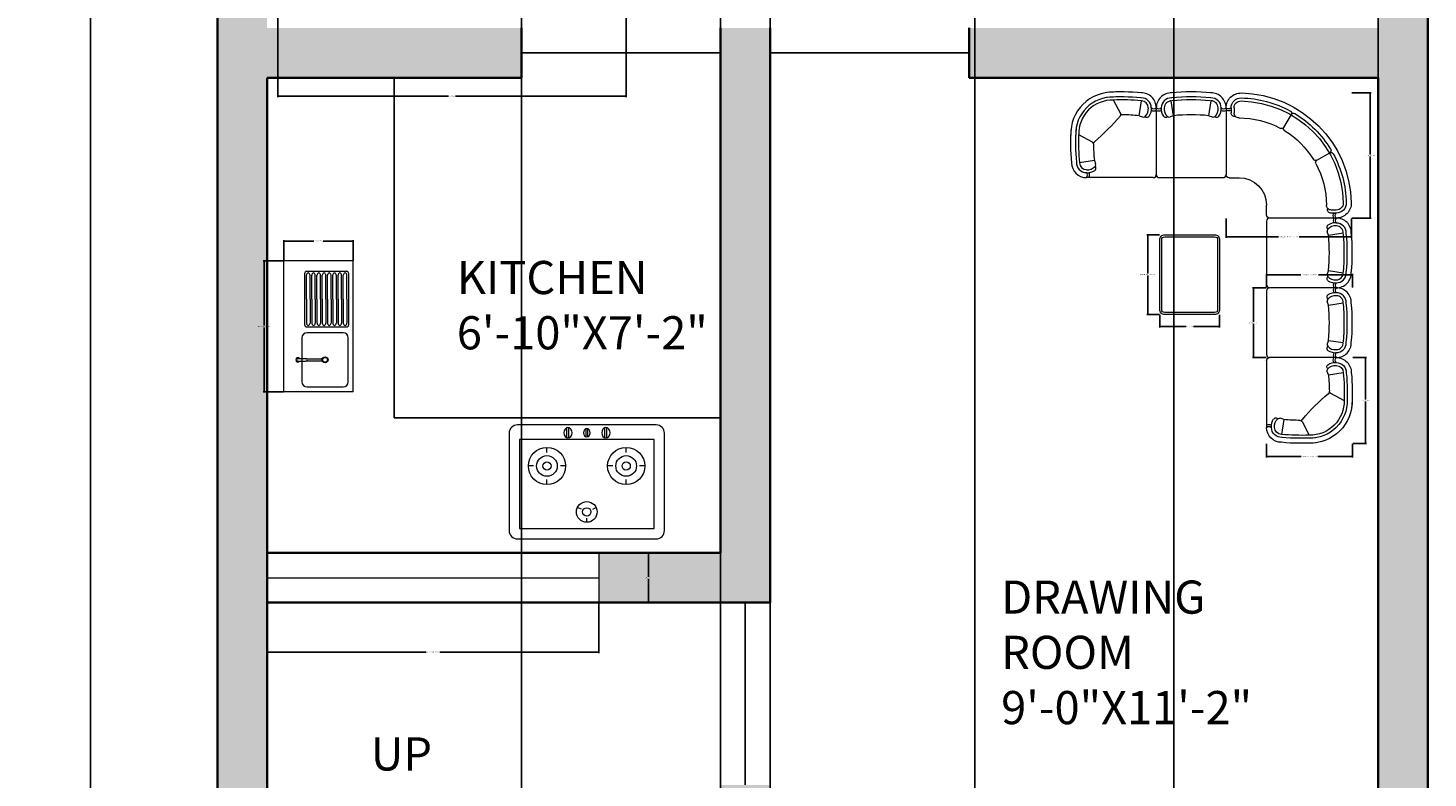
# Model space of a CAD drawing. Units: inches. Extents: x -16 to 587, y -783 to 64.
# Tile 7 of 14: x -16 to 237, y -527 to -392. Entities that reach past the tile are written whole.
import ezdxf

# ---------------------------------------------------------------- set-up
doc = ezdxf.new("R2010")
doc.units = ezdxf.units.IN
doc.header["$MEASUREMENT"] = 0
for name, color, linetype, lineweight in [('A-ANNO-DIMS', 2, 'Continuous', 18), ('A-ANNO-TEXT', 7, 'Continuous', 25), ('A-AREA-IDEN', 7, 'Continuous', 18), ('A-DOOR', 3, 'Continuous', 25), ('A-EQPM', 8, 'Continuous', 18), ('A-FLOR-CASE', 7, 'Continuous', 25), ('A-FLOR-FIXT', 9, 'Continuous', 18), ('A-FURN', 8, 'Continuous', 18), ('A-GLAZ', 4, 'Continuous', 18), ('A-WALL', 7, 'Continuous', 35), ('A-WALL-PATT', 23, 'Continuous', 13)]:
    doc.layers.add(name, color=color, linetype=linetype, lineweight=lineweight)
doc.styles.get("Standard").update_dxf_attribs({"font": 'arial.ttf'})
doc.dimstyles.get("Standard").update_dxf_attribs({"dimtxt": 0.18, "dimasz": 0.18, "dimexe": 0.18, "dimexo": 0.0625, "dimgap": 0.09, "dimtad": 0, "dimtih": 1, "dimtoh": 1, "dimdec": 0, "dimzin": 0, "dimdsep": 46, "dimlunit": 3, "dimtxsty": 'Standard', "dimcen": 0.09, "dimadec": 0, "dimazin": 0, "dimtfac": 1, "dimtdec": 0, "dimtofl": 0, "dimtmove": 0, "dimatfit": 3, "dimfxl": 1, "dimtolj": 1, "dimtzin": 0, "dimarcsym": 0})

# ---------------------------------------------------------------- blocks, each defined once
blk = doc.blocks.new('A$C707258B2')
at = {"color": 0}
for p, q in [((0.404, 0.342), (1.074, 0.342)), ((0.404, 0.292), (0.454, 0.292)), ((1.104, 0.312), (1.104, 0.212)), ((0.404, 0.262), (0.454, 0.262)), ((1.479, -0.063), (1.379, -0.063)), ((1.509, -0.763), (1.509, -0.093)), ((0.6, -0.238), (0.47, -0.313)), ((0.929, -0.567), (0.854, -0.697)), ((1.429, -0.763), (1.429, -0.713)), ((1.459, -0.763), (1.459, -0.712))]:
    blk.add_line(p, q, dxfattribs=at)
for centre, radius, start, end in [((0.404, 0.192), 0.15, 90, 181.1754), ((0.404, 0.192), 0.1, 90, 181.1754), ((0.378, 0.317), 0.0362, 316.3972, 43.6028), ((0.368, 0.317), 0.0662, 337.8298, 22.1702), ((0.455, 0.256), 0.0357, 345.4262, 90.5555), ((1.074, 0.312), 0.03, 360, 90), ((1.379, 0.212), 1.125, 181.1754, 268.8246), ((1.379, 0.212), 1.075, 181.1754, 208.6357), ((0.404, 0.192), 0.07, 90, 181.1754), ((1.379, 0.212), 1.045, 181.1754, 268.8246), ((0.454, 0.212), 0.05, 360, 90), ((1.379, 0.212), 0.875, 180, 208.4082), ((1.379, 0.212), 0.275, 180, 270), ((1.479, -0.093), 0.03, 360, 90), ((0.587, -0.216), 0.025, 300, 28.4082), ((0.612, -0.259), 0.025, 31.5918, 120), ((1.379, 0.212), 0.875, 211.5918, 238.4082), ((0.457, -0.291), 0.025, 208.6357, 300), ((0.482, -0.334), 0.025, 120, 211.3643), ((1.379, 0.212), 1.075, 211.3643, 238.6357), ((0.907, -0.555), 0.025, 330, 58.4082), ((0.951, -0.58), 0.025, 61.5918, 150), ((1.379, 0.212), 0.875, 241.5918, 270), ((0.832, -0.685), 0.025, 238.6357, 330), ((0.876, -0.71), 0.025, 150, 241.3643), ((1.379, -0.713), 0.05, 360, 90), ((1.425, -0.709), 0.0336, 354.6301, 109.3883), ((1.379, 0.212), 1.075, 241.3643, 268.8246), ((1.359, -0.763), 0.15, 268.8246, 360), ((1.359, -0.763), 0.1, 268.8246, 360), ((1.359, -0.763), 0.07, 268.8246, 360), ((1.484, -0.799), 0.0662, 67.8298, 112.1702), ((1.484, -0.789), 0.0362, 46.3972, 133.6028)]:
    blk.add_arc(centre, radius, start, end, dxfattribs=at)
blk = doc.blocks.new('A$C1352')
at = {"color": 0}
for points in [[(0.003, 0.053), (0.003, 0.553, -0.414214), (0.053, 0.603), (0.753, 0.603, -0.414214), (0.803, 0.553), (0.803, 0.053, -0.414214), (0.753, 0.003), (0.053, 0.003, -0.414214)], [(0.023, 0.053), (0.023, 0.553, -0.414214), (0.053, 0.583), (0.753, 0.583, -0.414214), (0.783, 0.553), (0.783, 0.053, -0.414214), (0.753, 0.023), (0.053, 0.023, -0.414214)]]:
    blk.add_lwpolyline(points, format="xyb", close=True, dxfattribs=at)
blk = doc.blocks.new('part 01')
at = {"color": 0}
for p, q in [((-670, 700), (0, 700)), ((30, 30), (30, 670)), ((-591, 527), (-740, 550)), ((-591, 527), (-579, 561)), ((-591, 173), (-740, 150)), ((-591, 173), (-579, 139)), ((-670, 0), (0, 0))]:
    blk.add_line(p, q, dxfattribs=at)
for centre, radius, start, end in [((-670, 550), 150, 90, 181.1754), ((-670, 550), 100, 90, 181.1754), ((-670, 550), 70, 90, 181.1754), ((-660, 518), 133, 56.0897, 95.6132), ((-696, 675), 36.2, 316.3972, 43.6028), ((-660, 518), 103, 42.0066, 95.6132), ((-706, 675), 66.2, 337.8298, 22.1702), ((-600, 607), 25, 332.9608, 56.0897), ((-625, 620), 53.2, 321.0017, 332.9608), ((-602, 570), 25, 340, 42.0066), ((0, 670), 30, 0, 90), ((1178, 350), 2008, 174.2835, 185.7165), ((1178, 350), 1958, 174.2835, 185.7165), ((1178, 350), 1928, 174.2835, 185.7165), ((1178, 350), 1778, 174.2835, 185.7165), ((-670, 150), 150, 178.8246, 270), ((-670, 150), 100, 178.8246, 270), ((-670, 150), 70, 178.8246, 270), ((-660, 182), 133, 264.3868, 303.9103), ((-660, 182), 103, 264.3868, 317.9934), ((-696, 25), 36.2, 316.3972, 43.6028), ((-706, 25), 66.2, 337.8298, 22.1702), ((-600, 93), 25, 303.9103, 27.0392), ((-602, 130), 25, 317.9934, 20), ((-625, 80), 53.2, 27.0392, 38.9983), ((0, 30), 30, 270, 0)]:
    blk.add_arc(centre, radius, start, end, dxfattribs=at)
blk = doc.blocks.new('part02')
at = {"color": 0}
for p, q in [((0, -670), (0, 0)), ((30, 30), (700, 30)), ((621, -143), (609, -109)), ((621, -143), (770, -120)), ((640, -326), (778, -399)), ((173, -591), (139, -579)), ((173, -591), (150, -740)), ((356, -610), (429, -748))]:
    blk.add_line(p, q, dxfattribs=at)
for centre, radius, start, end in [((30, 0), 30, 90, 180), ((726, 5), 56.2, 153.6122, 206.6666), ((726, 5), 36.2, 136.3972, 223.6028), ((700, -120), 150, 0, 90), ((630, -63), 25, 123.9103, 207.0392), ((655, -50), 53.2, 207.0392, 218.9983), ((632, -100), 25, 137.9934, 200), ((690, -152), 103, 84.3868, 137.9934), ((689, -151), 132, 85.4378, 123.9887), ((700, -121), 101, 357.5006, 89.858), ((700, -120), 70, 0, 90), ((-1228, -320), 2008, 357.7349, 5.7032), ((-1148, -320), 1958, 355.8657, 5.7165), ((-1148, -320), 2008, 355.818, 5.7165), ((-1148, -320), 1778, 0.3836, 5.7165), ((2220, -2190), 2454, 130.6961, 139.3039), ((439, -409), 419, 268.2181, 1.7819), ((439, -409), 369, 268.2181, 1.7819), ((439, -409), 339, 268.2181, 1.7819), ((632, -344), 20, 62, 130.6961), ((650, -308), 20, 180.3836, 242), ((25, -696), 56.2, 63.3334, 116.3878), ((25, -696), 36.2, 46.3972, 133.6028), ((150, -670), 150, 180, 271.1754), ((182, -660), 133, 146.0897, 185.6132), ((150, -670), 100, 180, 271.1754), ((93, -600), 25, 62.9608, 146.0897), ((182, -660), 103, 132.0066, 185.6132), ((150, -670), 70, 180, 270), ((80, -625), 53.2, 51.0017, 62.9608), ((130, -602), 25, 70, 132.0066), ((350, 1178), 1778, 264.2835, 269.6164), ((338, -620), 20, 28, 89.6164), ((374, -602), 20, 139.3039, 208), ((350, 1258), 2008, 264.2968, 272.2651), ((350, 1178), 2008, 264.2835, 274.182), ((350, 1178), 1958, 264.2835, 274.1343)]:
    blk.add_arc(centre, radius, start, end, dxfattribs=at)
blk = doc.blocks.new('*D6')
at = {"layer": 'A-ANNO-DIMS', "color": 0, "lineweight": -2, "transparency": 16777216}
for p, q in [((18.02, 19.45), (-5.05, 19.45)), ((-4.87, 19.27), (-4.87, -355.9)), ((-4.87, -737.37), (-4.87, -362.21)), ((18.02, -737.55), (-5.05, -737.55))]:
    blk.add_line(p, q, dxfattribs=at)
at = {"layer": 'A-ANNO-DIMS', "color": 0, "transparency": 16777216}
for points in [[(-4.9, 19.27), (-4.84, 19.27), (-4.87, 19.45)], [(-4.9, -737.37), (-4.84, -737.37), (-4.87, -737.55)]]:
    blk.add_solid(points, dxfattribs=at)
at = {"layer": 'Defpoints', "color": 0, "transparency": 16777216}
for p in [(18.08, 19.45), (-4.87, -737.55), (18.08, -737.55)]:
    blk.add_point(p, dxfattribs=at)
at = {"layer": 'A-ANNO-DIMS', "color": 0, "transparency": 16777216, "insert": (-4.87, -359.05), "char_height": 6, "attachment_point": 5}
blk.add_mtext('\\A1;63\'-1"', dxfattribs=at)
blk = doc.blocks.new('KITCHEN-SINK')
for p, q in [((12.53, 23.71), (0, 23.71)), ((0, 0), (0, 23.71)), ((12.53, 0), (12.53, 23.71)), ((3.76, 21.39), (3.76, 12.19)), ((4.1, 16.79), (4.1, 21.13)), ((4.19, 21.83), (11.32, 21.83)), ((4.75, 16.79), (4.75, 21.13)), ((5.05, 16.79), (5.05, 21.13)), ((5.7, 16.79), (5.7, 21.13)), ((6, 16.79), (6, 21.13)), ((6.65, 16.79), (6.65, 21.13)), ((6.96, 16.79), (6.96, 21.13)), ((7.6, 16.79), (7.6, 21.13)), ((7.91, 16.79), (7.91, 21.13)), ((8.56, 16.79), (8.56, 21.13)), ((8.86, 16.79), (8.86, 21.13)), ((9.51, 16.79), (9.51, 21.13)), ((9.81, 16.79), (9.81, 21.13)), ((10.46, 16.79), (10.46, 21.13)), ((10.76, 16.79), (10.76, 21.13)), ((11.41, 16.79), (11.41, 21.13)), ((11.75, 12.19), (11.75, 21.39)), ((4.1, 16.79), (4.1, 12.45)), ((4.75, 16.79), (4.75, 12.45)), ((5.05, 16.79), (5.05, 12.45)), ((5.7, 16.79), (5.7, 12.45)), ((6, 16.79), (6, 12.45)), ((6.65, 16.79), (6.65, 12.45)), ((6.96, 16.79), (6.96, 12.45)), ((7.6, 16.79), (7.6, 12.45)), ((7.91, 16.79), (7.91, 12.45)), ((8.56, 16.79), (8.56, 12.45)), ((8.86, 16.79), (8.86, 12.45)), ((9.51, 16.79), (9.51, 12.45)), ((9.81, 16.79), (9.81, 12.45)), ((10.46, 16.79), (10.46, 12.45)), ((10.76, 16.79), (10.76, 12.45)), ((11.41, 16.79), (11.41, 12.45)), ((4.19, 11.76), (11.32, 11.76)), ((10.73, 10.7), (4.21, 10.7)), ((3.28, 9.77), (3.28, 6.06)), ((11.66, 1.84), (11.66, 9.77)), ((3.28, 5.95), (3.28, 1.84)), ((4.21, 0.91), (10.73, 0.91)), ((12.53, 0), (0, 0))]:
    blk.add_line(p, q)
for points in [[(2.55, 6.06), (3.98, 6.06)], [(2.55, 5.54), (3.98, 5.54)], [(4.14, 6), (6.76, 6)], [(4.14, 5.61), (6.76, 5.61)]]:
    blk.add_lwpolyline(points)
for radius in [0.54, 0.432]:
    blk.add_circle((7.47, 5.8), radius)
for centre, radius, start, end in [((4.19, 21.39), 0.432, 90, 180), ((4.53, 21.13), 0.432, 104.4903, 180), ((4.32, 21.13), 0.432, 0, 75.5097), ((5.48, 21.13), 0.432, 104.4903, 180), ((5.27, 21.13), 0.432, 0, 75.5097), ((6.44, 21.13), 0.432, 104.4903, 180), ((6.22, 21.13), 0.432, 0, 75.5097), ((7.39, 21.13), 0.432, 104.4903, 180), ((7.17, 21.13), 0.432, 0, 75.5097), ((8.34, 21.13), 0.432, 104.4903, 180), ((8.12, 21.13), 0.432, 0, 75.5097), ((9.29, 21.13), 0.432, 104.4903, 180), ((9.07, 21.13), 0.432, 0, 75.5097), ((10.24, 21.13), 0.432, 104.4903, 180), ((10.03, 21.13), 0.432, 0, 75.5097), ((11.19, 21.13), 0.432, 104.4903, 180), ((10.98, 21.13), 0.432, 0, 75.5097), ((11.32, 21.39), 0.432, 0, 90), ((4.21, 9.77), 0.933, 90, 180), ((4.19, 12.19), 0.432, 180, 270), ((4.53, 12.45), 0.432, 180, 255.5097), ((4.32, 12.45), 0.432, 284.4903, 0), ((5.48, 12.45), 0.432, 180, 255.5097), ((5.27, 12.45), 0.432, 284.4903, 0), ((6.44, 12.45), 0.432, 180, 255.5097), ((6.22, 12.45), 0.432, 284.4903, 0), ((7.39, 12.45), 0.432, 180, 255.5097), ((7.17, 12.45), 0.432, 284.4903, 0), ((8.34, 12.45), 0.432, 180, 255.5097), ((8.12, 12.45), 0.432, 284.4903, 0), ((9.29, 12.45), 0.432, 180, 255.5097), ((9.07, 12.45), 0.432, 284.4903, 0), ((10.24, 12.45), 0.432, 180, 255.5097), ((10.03, 12.45), 0.432, 284.4903, 0), ((10.73, 9.77), 0.933, 0, 90), ((11.19, 12.45), 0.432, 180, 255.5097), ((10.98, 12.45), 0.432, 284.4903, 0), ((11.32, 12.19), 0.432, 270, 0), ((2.55, 5.8), 0.388, 41.9018, 318.0982), ((2.55, 5.8), 0.259, 90, 270), ((3.97, 5.8), 0.259, 272.2198, 87.7802), ((6.78, 5.8), 0.195, 264.9463, 95.0537), ((4.21, 1.84), 0.933, 180, 270), ((10.73, 1.84), 0.933, 270, 0)]:
    blk.add_arc(centre, radius, start, end)
blk = doc.blocks.new('COOKTOP-THREE-BURNER')
for p, q in [((26.61, 20.61), (1.5, 20.61)), ((0, 19.11), (0, 1.5)), ((26.23, 17.99), (1.87, 17.99)), ((1.87, 17.99), (1.87, 1.87)), ((10.46, 18.28), (10.46, 20.15)), ((10.83, 18.28), (10.83, 20.15)), ((13.92, 18.45), (13.92, 19.97)), ((14.22, 18.45), (14.22, 19.97)), ((17.32, 18.28), (17.32, 20.15)), ((17.7, 18.28), (17.7, 20.15)), ((26.23, 1.87), (26.23, 17.99)), ((28.11, 1.5), (28.11, 19.11)), ((6.85, 15.63), (6.85, 16.56)), ((21.18, 15.63), (21.18, 16.56)), ((4.42, 13.19), (3.48, 13.19)), ((10.23, 13.19), (9.29, 13.19)), ((18.74, 13.19), (17.8, 13.19)), ((24.55, 13.19), (23.61, 13.19)), ((6.85, 9.82), (6.85, 10.76)), ((21.18, 9.82), (21.18, 10.76)), ((12.37, 5.69), (13.06, 5.41)), ((15.74, 5.69), (15.08, 5.34)), ((14.05, 3), (14.05, 3.75)), ((1.5, 0), (26.61, 0)), ((1.87, 1.87), (26.23, 1.87))]:
    blk.add_line(p, q)
for centre, radius in [((6.85, 13.19), 3.37), ((21.18, 13.19), 3.37), ((6.85, 13.19), 1.87), ((6.85, 13.19), 0.75), ((21.18, 13.19), 1.87), ((21.18, 13.19), 0.75), ((14.05, 4.88), 1.87), ((14.05, 4.88), 0.75)]:
    blk.add_circle(centre, radius)
for centre, start, end in [((1.5, 19.11), 90, 180), ((26.61, 19.11), 0, 90), ((1.5, 1.5), 180, 270), ((26.61, 1.5), 270, 0)]:
    blk.add_arc(centre, 1.5, start, end)
at = {"extrusion": (0, 0, -1)}
for centre, major_axis in [((10.65, 19.21), (0, 0.937)), ((14.07, 19.21), (0, 0.759)), ((17.51, 19.21), (0, 0.937))]:
    blk.add_ellipse(centre, major_axis=major_axis, ratio=0.802399, dxfattribs=at)
blk = doc.blocks.new('WIN-60')
for p, q in [((0, 9), (60, 9)), ((0, 0), (0, 9)), ((60, 9), (60, 0)), ((0, 4.5), (60, 4.5)), ((60, 0), (0, 0))]:
    blk.add_line(p, q)
blk = doc.blocks.new('*D20')
at = {"layer": 'A-ANNO-DIMS', "color": 0, "lineweight": -2, "transparency": 16777216}
for p, q in [((207.87, -438.52), (207.87, -436.07)), ((208.05, -436.25), (214.07, -436.25)), ((223.26, -436.25), (217.25, -436.25)), ((223.44, -438.52), (223.44, -436.07))]:
    blk.add_line(p, q, dxfattribs=at)
at = {"layer": 'A-ANNO-DIMS', "color": 0, "transparency": 16777216}
for points in [[(208.05, -436.22), (208.05, -436.28), (207.87, -436.25)], [(223.26, -436.22), (223.26, -436.28), (223.44, -436.25)]]:
    blk.add_solid(points, dxfattribs=at)
at = {"layer": 'Defpoints', "color": 0, "transparency": 16777216}
for p in [(207.87, -436.25), (207.87, -438.58), (223.44, -438.58)]:
    blk.add_point(p, dxfattribs=at)
at = {"layer": 'A-ANNO-DIMS', "color": 0, "transparency": 16777216, "insert": (215.66, -436.25), "char_height": 0.18, "attachment_point": 5}
blk.add_mtext('\\A1;SOFA SEAT 1\'-3 1/2" TYP.', dxfattribs=at)
blk = doc.blocks.new('*D21')
at = {"layer": 'A-ANNO-DIMS', "color": 0, "lineweight": -2, "transparency": 16777216}
for p, q in [((207.81, -438.58), (205.35, -438.58)), ((205.53, -438.76), (205.53, -444.72)), ((205.53, -451.03), (205.53, -445.08)), ((207.81, -451.21), (205.35, -451.21))]:
    blk.add_line(p, q, dxfattribs=at)
at = {"layer": 'A-ANNO-DIMS', "color": 0, "transparency": 16777216}
for points in [[(205.5, -438.76), (205.56, -438.76), (205.53, -438.58)], [(205.5, -451.03), (205.56, -451.03), (205.53, -451.21)]]:
    blk.add_solid(points, dxfattribs=at)
at = {"layer": 'Defpoints', "color": 0, "transparency": 16777216}
for p in [(207.87, -438.58), (205.53, -451.21), (207.87, -451.21)]:
    blk.add_point(p, dxfattribs=at)
at = {"layer": 'A-ANNO-DIMS', "color": 0, "transparency": 16777216, "insert": (205.53, -444.9), "char_height": 0.18, "attachment_point": 5}
blk.add_mtext('\\A1;1\'-0 1/2" TYP.', dxfattribs=at)
blk = doc.blocks.new('*D22')
at = {"layer": 'A-ANNO-DIMS', "color": 0, "lineweight": -2, "transparency": 16777216}
for p, q in [((207.87, -466.85), (207.87, -469.3)), ((223.44, -466.85), (223.44, -469.3)), ((208.05, -469.12), (214.13, -469.12)), ((223.26, -469.12), (217.18, -469.12))]:
    blk.add_line(p, q, dxfattribs=at)
at = {"layer": 'A-ANNO-DIMS', "color": 0, "transparency": 16777216}
for points in [[(208.05, -469.09), (208.05, -469.15), (207.87, -469.12)], [(223.26, -469.09), (223.26, -469.15), (223.44, -469.12)]]:
    blk.add_solid(points, dxfattribs=at)
at = {"layer": 'Defpoints', "color": 0, "transparency": 16777216}
for p in [(207.87, -466.78), (223.44, -466.78), (207.87, -469.12)]:
    blk.add_point(p, dxfattribs=at)
at = {"layer": 'A-ANNO-DIMS', "color": 0, "transparency": 16777216, "insert": (215.65, -469.12), "char_height": 0.18, "attachment_point": 5}
blk.add_mtext('\\A1;SOFA END 1\'-3 1/2" TYP.', dxfattribs=at)
blk = doc.blocks.new('*D23')
at = {"layer": 'A-ANNO-DIMS', "color": 0, "lineweight": -2, "transparency": 16777216}
for p, q in [((223.5, -451.21), (225.95, -451.21)), ((225.77, -451.39), (225.77, -458.82)), ((225.77, -466.6), (225.77, -459.18)), ((223.5, -466.78), (225.95, -466.78))]:
    blk.add_line(p, q, dxfattribs=at)
at = {"layer": 'A-ANNO-DIMS', "color": 0, "transparency": 16777216}
for points in [[(225.74, -451.39), (225.8, -451.39), (225.77, -451.21)], [(225.74, -466.6), (225.8, -466.6), (225.77, -466.78)]]:
    blk.add_solid(points, dxfattribs=at)
at = {"layer": 'Defpoints', "color": 0, "transparency": 16777216}
for p in [(223.44, -451.21), (223.44, -466.78), (225.77, -466.78)]:
    blk.add_point(p, dxfattribs=at)
at = {"layer": 'A-ANNO-DIMS', "color": 0, "transparency": 16777216, "insert": (225.77, -459), "char_height": 0.18, "attachment_point": 5}
blk.add_mtext('\\A1;1\'-3 1/2" TYP.', dxfattribs=at)
blk = doc.blocks.new('*D24')
at = {"layer": 'A-ANNO-DIMS', "color": 0, "lineweight": -2, "transparency": 16777216}
for p, q in [((200.56, -426.02), (200.56, -429.53)), ((223.22, -426.02), (223.22, -429.53)), ((200.74, -429.35), (210.02, -429.35)), ((223.04, -429.35), (213.76, -429.35))]:
    blk.add_line(p, q, dxfattribs=at)
at = {"layer": 'A-ANNO-DIMS', "color": 0, "transparency": 16777216}
for points in [[(200.74, -429.32), (200.74, -429.38), (200.56, -429.35)], [(223.04, -429.32), (223.04, -429.38), (223.22, -429.35)]]:
    blk.add_solid(points, dxfattribs=at)
at = {"layer": 'Defpoints', "color": 0, "transparency": 16777216}
for p in [(200.56, -425.95), (223.22, -425.95), (200.56, -429.35)]:
    blk.add_point(p, dxfattribs=at)
at = {"layer": 'A-ANNO-DIMS', "color": 0, "transparency": 16777216, "insert": (211.89, -429.35), "char_height": 0.18, "attachment_point": 5}
blk.add_mtext('\\A1;SOFA CORNER 1\'-10 1/2" TYP.', dxfattribs=at)
blk = doc.blocks.new('*D25')
at = {"layer": 'A-ANNO-DIMS', "color": 0, "lineweight": -2, "transparency": 16777216}
for p, q in [((223.28, -403.3), (226.8, -403.3)), ((226.62, -403.48), (226.62, -414.44)), ((226.62, -425.77), (226.62, -414.81)), ((223.28, -425.95), (226.8, -425.95))]:
    blk.add_line(p, q, dxfattribs=at)
at = {"layer": 'A-ANNO-DIMS', "color": 0, "transparency": 16777216}
for points in [[(226.59, -403.48), (226.65, -403.48), (226.62, -403.3)], [(226.59, -425.77), (226.65, -425.77), (226.62, -425.95)]]:
    blk.add_solid(points, dxfattribs=at)
at = {"layer": 'Defpoints', "color": 0, "transparency": 16777216}
for p in [(223.22, -403.3), (223.22, -425.95), (226.62, -425.95)]:
    blk.add_point(p, dxfattribs=at)
at = {"layer": 'A-ANNO-DIMS', "color": 0, "transparency": 16777216, "insert": (226.62, -414.63), "char_height": 0.18, "attachment_point": 5}
blk.add_mtext('\\A1;1\'-10 1/2" TYP.', dxfattribs=at)
blk = doc.blocks.new('*D26')
at = {"layer": 'A-ANNO-DIMS', "color": 0, "lineweight": -2, "transparency": 16777216}
for p, q in [((188.49, -428.98), (186.21, -428.98)), ((186.39, -429.16), (186.39, -436.01)), ((186.39, -443.23), (186.39, -436.38)), ((188.49, -443.41), (186.21, -443.41))]:
    blk.add_line(p, q, dxfattribs=at)
at = {"layer": 'A-ANNO-DIMS', "color": 0, "transparency": 16777216}
for points in [[(186.36, -429.16), (186.42, -429.16), (186.39, -428.98)], [(186.36, -443.23), (186.42, -443.23), (186.39, -443.41)]]:
    blk.add_solid(points, dxfattribs=at)
at = {"layer": 'Defpoints', "color": 0, "transparency": 16777216}
for p in [(188.55, -428.98), (186.39, -443.41), (188.55, -443.41)]:
    blk.add_point(p, dxfattribs=at)
at = {"layer": 'A-ANNO-DIMS', "color": 0, "transparency": 16777216, "insert": (186.39, -436.2), "char_height": 0.18, "attachment_point": 5}
blk.add_mtext('\\A1;SIDE TABLE 1\'-2 1/2" TYP.', dxfattribs=at)
blk = doc.blocks.new('*D27')
at = {"layer": 'A-ANNO-DIMS', "color": 0, "lineweight": -2, "transparency": 16777216}
for p, q in [((188.55, -443.48), (188.55, -445.76)), ((188.73, -445.58), (193.26, -445.58)), ((199.2, -445.58), (194.68, -445.58)), ((199.38, -443.48), (199.38, -445.76))]:
    blk.add_line(p, q, dxfattribs=at)
at = {"layer": 'A-ANNO-DIMS', "color": 0, "transparency": 16777216}
for points in [[(188.73, -445.55), (188.73, -445.61), (188.55, -445.58)], [(199.2, -445.55), (199.2, -445.61), (199.38, -445.58)]]:
    blk.add_solid(points, dxfattribs=at)
at = {"layer": 'Defpoints', "color": 0, "transparency": 16777216}
for p in [(188.55, -443.41), (199.38, -443.41), (199.38, -445.58)]:
    blk.add_point(p, dxfattribs=at)
at = {"layer": 'A-ANNO-DIMS', "color": 0, "transparency": 16777216, "insert": (193.97, -445.58), "char_height": 0.18, "attachment_point": 5}
blk.add_mtext('\\A1;0\'-11" TYP.', dxfattribs=at)
blk = doc.blocks.new('*D37')
at = {"layer": 'A-ANNO-DIMS', "color": 0, "lineweight": -2, "transparency": 16777216}
for p, q in [((29.02, -389.37), (29.02, -404.05)), ((92.05, -389.37), (92.05, -404.05)), ((29.2, -403.87), (59.9, -403.87)), ((91.87, -403.87), (61.18, -403.87))]:
    blk.add_line(p, q, dxfattribs=at)
at = {"layer": 'A-ANNO-DIMS', "color": 0, "transparency": 16777216}
for points in [[(29.2, -403.84), (29.2, -403.9), (29.02, -403.87)], [(91.87, -403.84), (91.87, -403.9), (92.05, -403.87)]]:
    blk.add_solid(points, dxfattribs=at)
at = {"layer": 'Defpoints', "color": 0, "transparency": 16777216}
for p in [(29.02, -389.31), (92.05, -389.31), (92.05, -403.87)]:
    blk.add_point(p, dxfattribs=at)
at = {"layer": 'A-ANNO-DIMS', "color": 0, "transparency": 16777216, "insert": (60.54, -403.87), "char_height": 0.18, "attachment_point": 5}
blk.add_mtext('\\A1;5\'-3" TYP.', dxfattribs=at)
blk = doc.blocks.new('*D38')
at = {"layer": 'A-ANNO-DIMS', "color": 0, "lineweight": -2, "transparency": 16777216}
for p, q in [((30.03, -433.72), (26.35, -433.72)), ((26.53, -433.9), (26.53, -445.39)), ((26.53, -457.24), (26.53, -445.75)), ((30.03, -457.42), (26.35, -457.42))]:
    blk.add_line(p, q, dxfattribs=at)
at = {"layer": 'A-ANNO-DIMS', "color": 0, "transparency": 16777216}
for points in [[(26.5, -433.9), (26.56, -433.9), (26.53, -433.72)], [(26.5, -457.24), (26.56, -457.24), (26.53, -457.42)]]:
    blk.add_solid(points, dxfattribs=at)
at = {"layer": 'Defpoints', "color": 0, "transparency": 16777216}
for p in [(26.53, -433.72), (30.09, -433.72), (30.09, -457.42)]:
    blk.add_point(p, dxfattribs=at)
at = {"layer": 'A-ANNO-DIMS', "color": 0, "transparency": 16777216, "insert": (26.53, -445.57), "char_height": 0.18, "attachment_point": 5}
blk.add_mtext('\\A1;SINK 1\'-11 1/2" TYP.', dxfattribs=at)
blk = doc.blocks.new('*D39')
at = {"layer": 'A-ANNO-DIMS', "color": 0, "lineweight": -2, "transparency": 16777216}
for p, q in [((30.09, -433.65), (30.09, -429.98)), ((30.27, -430.16), (35.52, -430.16)), ((42.44, -430.16), (37.2, -430.16)), ((42.62, -433.65), (42.62, -429.98))]:
    blk.add_line(p, q, dxfattribs=at)
at = {"layer": 'A-ANNO-DIMS', "color": 0, "transparency": 16777216}
for points in [[(30.27, -430.13), (30.27, -430.19), (30.09, -430.16)], [(42.44, -430.13), (42.44, -430.19), (42.62, -430.16)]]:
    blk.add_solid(points, dxfattribs=at)
at = {"layer": 'Defpoints', "color": 0, "transparency": 16777216}
for p in [(42.62, -430.16), (30.09, -433.72), (42.62, -433.72)]:
    blk.add_point(p, dxfattribs=at)
at = {"layer": 'A-ANNO-DIMS', "color": 0, "transparency": 16777216, "insert": (36.36, -430.16), "char_height": 0.18, "attachment_point": 5}
blk.add_mtext('\\A1;1\'-0 1/2" TYP.', dxfattribs=at)
blk = doc.blocks.new('*D46')
at = {"layer": 'A-ANNO-DIMS', "color": 0, "lineweight": -2, "transparency": 16777216}
for p, q in [((27.08, -495.62), (27.08, -504.73)), ((87.08, -495.62), (87.08, -504.73)), ((27.26, -504.55), (55.85, -504.55)), ((86.9, -504.55), (58.31, -504.55))]:
    blk.add_line(p, q, dxfattribs=at)
at = {"layer": 'A-ANNO-DIMS', "color": 0, "transparency": 16777216}
for points in [[(27.26, -504.52), (27.26, -504.58), (27.08, -504.55)], [(86.9, -504.52), (86.9, -504.58), (87.08, -504.55)]]:
    blk.add_solid(points, dxfattribs=at)
at = {"layer": 'Defpoints', "color": 0, "transparency": 16777216}
for p in [(27.08, -495.55), (87.08, -495.55), (87.08, -504.55)]:
    blk.add_point(p, dxfattribs=at)
at = {"layer": 'A-ANNO-DIMS', "color": 0, "transparency": 16777216, "insert": (57.08, -504.55), "char_height": 0.18, "attachment_point": 5}
blk.add_mtext('\\A1;WINDOW 5\'-0" TYP.', dxfattribs=at)
blk = doc.blocks.new('*D47')
at = {"layer": 'A-ANNO-DIMS', "color": 0, "lineweight": -2, "transparency": 16777216}
for p, q in [((87.15, -486.55), (96.26, -486.55)), ((96.08, -486.73), (96.08, -490.87)), ((96.08, -495.37), (96.08, -491.24)), ((87.15, -495.55), (96.26, -495.55))]:
    blk.add_line(p, q, dxfattribs=at)
at = {"layer": 'A-ANNO-DIMS', "color": 0, "transparency": 16777216}
for points in [[(96.05, -486.73), (96.11, -486.73), (96.08, -486.55)], [(96.05, -495.37), (96.11, -495.37), (96.08, -495.55)]]:
    blk.add_solid(points, dxfattribs=at)
at = {"layer": 'Defpoints', "color": 0, "transparency": 16777216}
for p in [(87.08, -486.55), (96.08, -486.55), (87.08, -495.55)]:
    blk.add_point(p, dxfattribs=at)
at = {"layer": 'A-ANNO-DIMS', "color": 0, "transparency": 16777216, "insert": (96.08, -491.05), "char_height": 0.18, "attachment_point": 5}
blk.add_mtext('\\A1;0\'-9" TYP.', dxfattribs=at)
blk = doc.blocks.new('*D56')
at = {"layer": 'A-ANNO-DIMS', "color": 0, "lineweight": -2, "transparency": 16777216}
for p, q in [((118.08, -728.49), (118.08, 63.78)), ((118.26, 63.6), (172.75, 63.6)), ((227.9, 63.6), (173.41, 63.6)), ((228.08, -728.49), (228.08, 63.78))]:
    blk.add_line(p, q, dxfattribs=at)
at = {"layer": 'A-ANNO-DIMS', "color": 0, "transparency": 16777216}
for points in [[(118.26, 63.63), (118.26, 63.57), (118.08, 63.6)], [(227.9, 63.63), (227.9, 63.57), (228.08, 63.6)]]:
    blk.add_solid(points, dxfattribs=at)
at = {"layer": 'Defpoints', "color": 0, "transparency": 16777216}
for p in [(228.08, 63.6), (118.08, -728.55), (228.08, -728.55)]:
    blk.add_point(p, dxfattribs=at)
at = {"layer": 'A-ANNO-DIMS', "color": 0, "transparency": 16777216, "insert": (173.08, 63.6), "char_height": 0.18, "attachment_point": 5}
blk.add_mtext('\\A1;9\'-2"', dxfattribs=at)
blk = doc.blocks.new('*D57')
at = {"layer": 'A-ANNO-DIMS', "color": 0, "lineweight": -2, "transparency": 16777216}
for p, q in [((155.08, -534.49), (155.08, 63.78)), ((155.26, 63.6), (172.75, 63.6)), ((190.9, 63.6), (173.41, 63.6)), ((191.08, -534.49), (191.08, 63.78))]:
    blk.add_line(p, q, dxfattribs=at)
at = {"layer": 'A-ANNO-DIMS', "color": 0, "transparency": 16777216}
for points in [[(155.26, 63.63), (155.26, 63.57), (155.08, 63.6)], [(190.9, 63.63), (190.9, 63.57), (191.08, 63.6)]]:
    blk.add_solid(points, dxfattribs=at)
at = {"layer": 'Defpoints', "color": 0, "transparency": 16777216}
for p in [(191.08, 63.6), (155.08, -534.55), (191.08, -534.55)]:
    blk.add_point(p, dxfattribs=at)
at = {"layer": 'A-ANNO-DIMS', "color": 0, "transparency": 16777216, "insert": (173.08, 63.6), "char_height": 0.18, "attachment_point": 5}
blk.add_mtext('\\A1;3\'-0"', dxfattribs=at)
blk = doc.blocks.new('*D58')
at = {"layer": 'A-ANNO-DIMS', "color": 0, "lineweight": -2, "transparency": 16777216}
for p, q in [((73.08, -663.49), (73.08, 63.78)), ((73.26, 63.6), (90.75, 63.6)), ((108.9, 63.6), (91.41, 63.6)), ((109.08, -667.99), (109.08, 63.78))]:
    blk.add_line(p, q, dxfattribs=at)
at = {"layer": 'A-ANNO-DIMS', "color": 0, "transparency": 16777216}
for points in [[(73.26, 63.63), (73.26, 63.57), (73.08, 63.6)], [(108.9, 63.63), (108.9, 63.57), (109.08, 63.6)]]:
    blk.add_solid(points, dxfattribs=at)
at = {"layer": 'Defpoints', "color": 0, "transparency": 16777216}
for p in [(109.08, 63.6), (73.08, -663.55), (109.08, -668.05)]:
    blk.add_point(p, dxfattribs=at)
at = {"layer": 'A-ANNO-DIMS', "color": 0, "transparency": 16777216, "insert": (91.08, 63.6), "char_height": 0.18, "attachment_point": 5}
blk.add_mtext('\\A1;3\'-0"', dxfattribs=at)

msp = doc.modelspace()

# ---------------------------------------------------------------- hatches: boundary and pattern name
at = {"layer": 'A-WALL-PATT'}
h = msp.add_hatch(color=256, dxfattribs=at)
h.dxf.hatch_style = 1
h.paths.add_polyline_path([(137.08, -543.55), (137.08, -534.55), (118.08, -534.55), (118.08, -528.55), (109.08, -528.55), (109.08, -534.55), (109.08, -672.55), (118.08, -672.55), (118.08, -543.55)], flags=17)
h.paths.add_polyline_path([(27.08, -663.55), (27.08, -400.55), (73.08, -400.55), (73.08, -391.55), (27.08, -391.55), (27.08, 10.45), (48.75, 10.45), (171.08, 10.45), (171.08, -17.55), (180.08, -17.55), (180.08, 10.45), (228.08, 10.45), (228.08, -262.55), (206.41, -262.55), (118.08, -262.55), (118.08, -271.55), (228.08, -271.55), (228.08, -391.55), (154.08, -391.55), (154.08, -400.55), (228.08, -400.55), (228.08, -534.55), (209.08, -534.55), (209.08, -543.55), (237.08, -543.55), (237.08, 19.45), (18.08, 19.45), (18.08, -672.55), (73.08, -672.55), (73.08, -663.55)])
h.paths.add_polyline_path([(109.08, -486.55), (87.08, -486.55), (87.08, -495.55), (118.08, -495.55), (118.08, -400.55), (118.08, -391.55), (109.08, -391.55), (109.08, -400.55)], flags=17)

# ---------------------------------------------------------------- linework, layer by layer
at = {"layer": 'A-DOOR'}
for p, q in [((73.08, -396.05), (109.08, -396.05)), ((118.08, -396.05), (154.08, -396.05)), ((113.58, -528.55), (113.58, -495.55))]:
    msp.add_line(p, q, dxfattribs=at)
at = {"layer": 'A-FLOR-CASE'}
for p, q in [((50.08, -400.55), (50.08, -462.09)), ((50.08, -462.09), (109.08, -462.09))]:
    msp.add_line(p, q, dxfattribs=at)
at = {"layer": 'A-WALL'}
for p, q in [((18.08, 19.45), (18.08, -737.55)), ((237.08, 19.45), (237.08, -737.55)), ((73.08, -391.55), (73.08, -400.55)), ((109.08, -400.55), (109.08, -391.55)), ((118.08, -400.55), (118.08, -391.55)), ((154.08, -391.55), (154.08, -400.55)), ((27.08, -400.55), (73.08, -400.55)), ((27.08, -400.55), (27.08, -663.55)), ((109.08, -400.55), (109.08, -486.55)), ((118.08, -400.55), (118.08, -495.55)), ((154.08, -400.55), (228.08, -400.55)), ((228.08, -400.55), (228.08, -534.55)), ((27.08, -486.55), (109.08, -486.55)), ((27.08, -495.55), (118.08, -495.55))]:
    msp.add_line(p, q, dxfattribs=at)

# ---------------------------------------------------------------- block references
at = {"layer": 'A-EQPM'}
msp.add_blockref('COOKTOP-THREE-BURNER', (70.85, -484.02), dxfattribs=at)
at = {"layer": 'A-FLOR-FIXT'}
msp.add_blockref('KITCHEN-SINK', (30.09, -457.42), dxfattribs=at)
at = {"layer": 'A-FURN', "ltscale": 0.03}
for name, p, xscale, yscale, zscale, rotation in [('part02', (187.93, -418.1), 0.0180440482994306, 0.0180440482994306, 0.0180440482994306, 180), ('part 01', (187.93, -418.1), 0.0180440482994306, 0.0180440482994306, 0.0180440482994306, 270), ('A$C707258B2', (206.73, -398.73), -18.04404829943058, 18.04404829943058, 18.04404829943058, 89.9999999999967), ('part 01', (208.41, -425.95), 0.0180440482994306, 0.0180440482994306, 0.0180440482994306, 180), ('A$C1352', (188.5, -428.93), 18.04404829943058, 18.04404829943058, 18.04404829943058, 270), ('part 01', (208.41, -438.58), 0.0180440482994306, 0.0180440482994306, 0.0180440482994306, 180), ('part02', (208.41, -451.21), -0.0180440482994306, 0.0180440482994306, 0.0180440482994306, 89.9999999999967)]:
    msp.add_blockref(name, p, dxfattribs=dict(at, xscale=xscale, yscale=yscale, zscale=zscale, rotation=rotation))
at = {"layer": 'A-GLAZ'}
msp.add_blockref('WIN-60', (27.08, -495.56), dxfattribs=at)

# ---------------------------------------------------------------- texts
at = {"layer": 'A-ANNO-TEXT', "insert": (45.82, -519.95), "char_height": 6, "attachment_point": 1}
msp.add_mtext('UP', dxfattribs=at)
at = {"layer": 'A-AREA-IDEN', "char_height": 6, "attachment_point": 1}
for s, insert in [('KITCHEN\\P6\'-10"X7\'-2"', (61.39, -433.72)), ('DRAWING\\PROOM\\P9\'-0"X11\'-2"', (159.86, -491.56))]:
    msp.add_mtext(s, dxfattribs=dict(at, insert=insert))

# ---------------------------------------------------------------- dimensions: what is measured, and where the dimension line sits
at = {"layer": 'A-ANNO-DIMS'}
for base, p1, p2, picture, middle in [((109.08, 63.6), (73.08, -663.55), (109.08, -668.05), '*D58', (91.08, 63.6)), ((228.08, 63.6), (118.08, -728.55), (228.08, -728.55), '*D56', (173.08, 63.6)), ((191.08, 63.6), (155.08, -534.55), (191.08, -534.55), '*D57', (173.08, 63.6))]:
    dim = msp.add_linear_dim(base=base, p1=p1, p2=p2, dimstyle='Standard', override={"dimdec": 1, "dimlfac": 1, "dimrnd": 0, "dimzin": 1, "dimdsep": 46, "dimlunit": 4, "dimfrac": 2}, dxfattribs=at)
    dim.commit()
    dim.dimension.update_dxf_attribs({"geometry": picture, "text_midpoint": middle})
dim = msp.add_linear_dim(base=(-4.87, -737.55), p1=(18.08, 19.45), p2=(18.08, -737.55), angle=90, dimstyle='Standard', override={"dimtxt": 6, "dimclrd": 0, "dimclre": 0, "dimclrt": 0}, dxfattribs=at)
dim.commit()
dim.dimension.update_dxf_attribs({"geometry": '*D6', "text_midpoint": (-4.87, -359.05)})
for base, p1, p2, text, picture, middle in [((92.05, -403.87), (29.02, -389.31), (92.05, -389.31), '<> TYP.', '*D37', (60.54, -403.87)), ((42.62, -430.16), (30.09, -433.72), (42.62, -433.72), '<> TYP.', '*D39', (36.36, -430.16)), ((199.38, -445.58), (188.55, -443.41), (199.38, -443.41), '<> TYP.', '*D27', (193.97, -445.58)), ((87.08, -504.55), (27.08, -495.55), (87.08, -495.55), 'WINDOW <> TYP.', '*D46', (57.08, -504.55))]:
    dim = msp.add_linear_dim(base=base, p1=p1, p2=p2, text=text, dimstyle='Standard', override={"dimdec": 1, "dimlfac": 1, "dimrnd": 0, "dimzin": 1, "dimdsep": 46, "dimlunit": 4, "dimfrac": 2}, dxfattribs=at)
    dim.commit()
    dim.dimension.update_dxf_attribs({"geometry": picture, "text_midpoint": middle})
for base, p1, p2, angle, text, picture, middle in [((226.6162, -425.9532), (223.2178, -403.2972), (223.2178, -425.9532), 270, '<> TYP.', '*D25', (226.6162, -414.6252)), ((200.56, -429.35), (223.22, -425.95), (200.56, -425.95), 180, 'SOFA CORNER <> TYP.', '*D24', (211.89, -429.35)), ((186.39, -443.41), (188.55, -428.98), (188.55, -443.41), 270, 'SIDE TABLE <> TYP.', '*D26', (186.39, -436.2)), ((26.53, -433.72), (30.09, -457.42), (30.09, -433.72), 90, 'SINK <> TYP.', '*D38', (26.53, -445.57)), ((207.87, -436.25), (223.44, -438.58), (207.87, -438.58), 180, 'SOFA SEAT <> TYP.', '*D20', (215.66, -436.25)), ((205.53, -451.21), (207.87, -438.58), (207.87, -451.21), 270, '<> TYP.', '*D21', (205.53, -444.9)), ((225.77, -466.78), (223.44, -451.21), (223.44, -466.78), 270, '<> TYP.', '*D23', (225.77, -459)), ((207.87, -469.12), (223.44, -466.78), (207.87, -466.78), 180, 'SOFA END <> TYP.', '*D22', (215.65, -469.12)), ((96.08, -486.55), (87.08, -495.55), (87.08, -486.55), 90, '<> TYP.', '*D47', (96.08, -491.05))]:
    dim = msp.add_linear_dim(base=base, p1=p1, p2=p2, angle=angle, text=text, dimstyle='Standard', override={"dimdec": 1, "dimlfac": 1, "dimrnd": 0, "dimzin": 1, "dimdsep": 46, "dimlunit": 4, "dimfrac": 2}, dxfattribs=at)
    dim.commit()
    dim.dimension.update_dxf_attribs({"geometry": picture, "text_midpoint": middle})

doc.saveas('drawing.dxf')
